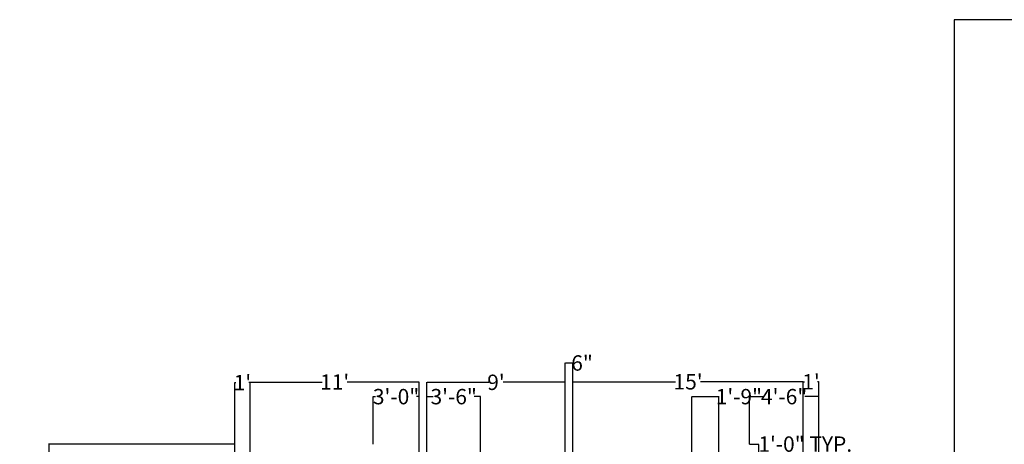
# Model space of a CAD drawing. Units: inches. Extents: x 2450 to 4494, y 1482 to 2597.
# Tile 3 of 7: x 2469 to 3238, y 2188 to 2519. Entities that reach past the tile are written whole.
import ezdxf

# ---------------------------------------------------------------- set-up
doc = ezdxf.new("R2010")
doc.units = ezdxf.units.IN
doc.header["$LTSCALE"] = 5
doc.header["$MEASUREMENT"] = 0
doc.layers.add('A-ANNO-DIMS', color=2, linetype='Continuous', lineweight=18)
doc.styles.get("Standard").update_dxf_attribs({"font": 'arial.ttf'})
doc.dimstyles.get("Standard").update_dxf_attribs({"dimtxt": 12, "dimasz": 0.18, "dimexe": 0.18, "dimexo": 0.0625, "dimgap": 0.09, "dimtad": 0, "dimtih": 1, "dimtoh": 1, "dimdec": 0, "dimzin": 0, "dimdsep": 46, "dimlunit": 3, "dimtxsty": 'Standard', "dimcen": 0.09, "dimadec": 0, "dimazin": 0, "dimtfac": 1, "dimtdec": 0, "dimtofl": 0, "dimtmove": 0, "dimatfit": 3, "dimfxl": 1, "dimtolj": 1, "dimtzin": 0, "dimarcsym": 0})

# ---------------------------------------------------------------- blocks, each defined once
blk = doc.blocks.new('*D6')
at = {"layer": 'A-ANNO-DIMS', "color": 0, "lineweight": -2, "ltscale": 5, "transparency": 16777216}
for p, q in [((2900.93, 2175.63), (2900.93, 2236.59)), ((2901.11, 2236.41), (2981.22, 2236.41)), ((3080.75, 2236.41), (3000.64, 2236.41)), ((3080.93, 2175.63), (3080.93, 2236.59))]:
    blk.add_line(p, q, dxfattribs=at)
at = {"layer": 'A-ANNO-DIMS', "color": 0, "ltscale": 5, "transparency": 16777216}
for points in [[(2901.11, 2236.44), (2901.11, 2236.38), (2900.93, 2236.41)], [(3080.75, 2236.44), (3080.75, 2236.38), (3080.93, 2236.41)]]:
    blk.add_solid(points, dxfattribs=at)
at = {"layer": 'Defpoints', "color": 0, "ltscale": 5, "transparency": 16777216}
for p in [(3080.93, 2236.41), (2900.93, 2175.57), (3080.93, 2175.57)]:
    blk.add_point(p, dxfattribs=at)
at = {"layer": 'A-ANNO-DIMS', "color": 0, "ltscale": 5, "transparency": 16777216, "insert": (2990.93, 2236.41), "char_height": 12, "attachment_point": 5}
blk.add_mtext("\\A1;15'", dxfattribs=at)
blk = doc.blocks.new('*D7')
at = {"layer": 'A-ANNO-DIMS', "color": 0, "lineweight": -2, "ltscale": 5, "transparency": 16777216}
for p, q in [((3080.93, 2175.63), (3080.93, 2236.59)), ((3081.11, 2236.41), (3081.88, 2236.41)), ((3092.75, 2236.41), (3091.98, 2236.41)), ((3092.93, 2175.63), (3092.93, 2236.59))]:
    blk.add_line(p, q, dxfattribs=at)
at = {"layer": 'A-ANNO-DIMS', "color": 0, "ltscale": 5, "transparency": 16777216}
for points in [[(3081.11, 2236.44), (3081.11, 2236.38), (3080.93, 2236.41)], [(3092.75, 2236.44), (3092.75, 2236.38), (3092.93, 2236.41)]]:
    blk.add_solid(points, dxfattribs=at)
at = {"layer": 'Defpoints', "color": 0, "ltscale": 5, "transparency": 16777216}
for p in [(3092.93, 2236.41), (3080.93, 2175.57), (3092.93, 2175.57)]:
    blk.add_point(p, dxfattribs=at)
at = {"layer": 'A-ANNO-DIMS', "color": 0, "ltscale": 5, "transparency": 16777216, "insert": (3086.93, 2236.41), "char_height": 12, "attachment_point": 5}
blk.add_mtext("\\A1;1'", dxfattribs=at)
blk = doc.blocks.new('*D8')
at = {"layer": 'A-ANNO-DIMS', "color": 0, "lineweight": -2, "ltscale": 5, "transparency": 16777216}
for p, q in [((2786.93, 2175.63), (2786.93, 2236.19)), ((2787.11, 2236.01), (2835.32, 2236.01)), ((2894.75, 2236.01), (2846.54, 2236.01)), ((2894.93, 2175.63), (2894.93, 2236.19))]:
    blk.add_line(p, q, dxfattribs=at)
at = {"layer": 'A-ANNO-DIMS', "color": 0, "ltscale": 5, "transparency": 16777216}
for points in [[(2787.11, 2236.04), (2787.11, 2235.98), (2786.93, 2236.01)], [(2894.75, 2236.04), (2894.75, 2235.98), (2894.93, 2236.01)]]:
    blk.add_solid(points, dxfattribs=at)
at = {"layer": 'Defpoints', "color": 0, "ltscale": 5, "transparency": 16777216}
for p in [(2894.93, 2236.01), (2786.93, 2175.57), (2894.93, 2175.57)]:
    blk.add_point(p, dxfattribs=at)
at = {"layer": 'A-ANNO-DIMS', "color": 0, "ltscale": 5, "transparency": 16777216, "insert": (2840.93, 2236.01), "char_height": 12, "attachment_point": 5}
blk.add_mtext("\\A1;9'", dxfattribs=at)
blk = doc.blocks.new('*D9')
at = {"layer": 'A-ANNO-DIMS', "color": 0, "lineweight": -2, "ltscale": 5, "transparency": 16777216}
for p, q in [((2894.93, 2175.63), (2894.93, 2251.28)), ((2895.11, 2251.1), (2900.75, 2251.1)), ((2900.93, 2175.63), (2900.93, 2251.28)), ((2900.93, 2251.1), (2901.11, 2251.1))]:
    blk.add_line(p, q, dxfattribs=at)
at = {"layer": 'A-ANNO-DIMS', "color": 0, "ltscale": 5, "transparency": 16777216}
for points in [[(2895.11, 2251.13), (2895.11, 2251.07), (2894.93, 2251.1)], [(2900.75, 2251.13), (2900.75, 2251.07), (2900.93, 2251.1)]]:
    blk.add_solid(points, dxfattribs=at)
at = {"layer": 'Defpoints', "color": 0, "ltscale": 5, "transparency": 16777216}
for p in [(2900.93, 2251.1), (2894.93, 2175.57), (2900.93, 2175.57)]:
    blk.add_point(p, dxfattribs=at)
at = {"layer": 'A-ANNO-DIMS', "color": 0, "ltscale": 5, "transparency": 16777216, "insert": (2908.13, 2251.1), "char_height": 12, "attachment_point": 5}
blk.add_mtext('\\A1;6"', dxfattribs=at)
blk = doc.blocks.new('*D10')
at = {"layer": 'A-ANNO-DIMS', "color": 0, "lineweight": -2, "ltscale": 5, "transparency": 16777216}
for p, q in [((2648.93, 2175.63), (2648.93, 2236.37)), ((2649.11, 2236.19), (2705.22, 2236.19)), ((2780.75, 2236.19), (2724.64, 2236.19)), ((2780.93, 2175.63), (2780.93, 2236.37))]:
    blk.add_line(p, q, dxfattribs=at)
at = {"layer": 'A-ANNO-DIMS', "color": 0, "ltscale": 5, "transparency": 16777216}
for points in [[(2649.11, 2236.22), (2649.11, 2236.16), (2648.93, 2236.19)], [(2780.75, 2236.22), (2780.75, 2236.16), (2780.93, 2236.19)]]:
    blk.add_solid(points, dxfattribs=at)
at = {"layer": 'Defpoints', "color": 0, "ltscale": 5, "transparency": 16777216}
for p in [(2780.93, 2236.19), (2648.93, 2175.57), (2780.93, 2175.57)]:
    blk.add_point(p, dxfattribs=at)
at = {"layer": 'A-ANNO-DIMS', "color": 0, "ltscale": 5, "transparency": 16777216, "insert": (2714.93, 2236.19), "char_height": 12, "attachment_point": 5}
blk.add_mtext("\\A1;11'", dxfattribs=at)
blk = doc.blocks.new('*D11')
at = {"layer": 'A-ANNO-DIMS', "color": 0, "lineweight": -2, "ltscale": 5, "transparency": 16777216}
for p, q in [((2636.93, 2175.63), (2636.93, 2235.95)), ((2637.11, 2235.77), (2637.88, 2235.77)), ((2648.75, 2235.77), (2647.98, 2235.77)), ((2648.93, 2175.63), (2648.93, 2235.95))]:
    blk.add_line(p, q, dxfattribs=at)
at = {"layer": 'A-ANNO-DIMS', "color": 0, "ltscale": 5, "transparency": 16777216}
for points in [[(2637.11, 2235.8), (2637.11, 2235.74), (2636.93, 2235.77)], [(2648.75, 2235.8), (2648.75, 2235.74), (2648.93, 2235.77)]]:
    blk.add_solid(points, dxfattribs=at)
at = {"layer": 'Defpoints', "color": 0, "ltscale": 5, "transparency": 16777216}
for p in [(2636.93, 2235.77), (2636.93, 2175.57), (2648.93, 2175.57)]:
    blk.add_point(p, dxfattribs=at)
at = {"layer": 'A-ANNO-DIMS', "color": 0, "ltscale": 5, "transparency": 16777216, "insert": (2642.93, 2235.77), "char_height": 12, "attachment_point": 5}
blk.add_mtext("\\A1;1'", dxfattribs=at)
blk = doc.blocks.new('*D41')
at = {"layer": 'A-ANNO-DIMS', "color": 0, "lineweight": -2, "ltscale": 5, "transparency": 16777216}
for p, q in [((2990.93, 2175.51), (2990.93, 2168.19)), ((2991.11, 2168.37), (3038.75, 2168.37)), ((3038.93, 2175.51), (3038.93, 2168.19)), ((3038.93, 2168.37), (3039.11, 2168.37))]:
    blk.add_line(p, q, dxfattribs=at)
at = {"layer": 'A-ANNO-DIMS', "color": 0, "ltscale": 5, "transparency": 16777216}
for points in [[(2991.11, 2168.4), (2991.11, 2168.34), (2990.93, 2168.37)], [(3038.75, 2168.4), (3038.75, 2168.34), (3038.93, 2168.37)]]:
    blk.add_solid(points, dxfattribs=at)
at = {"layer": 'Defpoints', "color": 0, "ltscale": 5, "transparency": 16777216}
for p in [(2990.93, 2175.57), (3038.93, 2175.57), (3038.93, 2168.37)]:
    blk.add_point(p, dxfattribs=at)
at = {"layer": 'A-ANNO-DIMS', "color": 0, "ltscale": 5, "transparency": 16777216, "insert": (3115.13, 2168.37), "char_height": 12, "attachment_point": 5}
blk.add_mtext('\\A1;WINDOW 4\'-0" TYP.', dxfattribs=at)
blk = doc.blocks.new('*D42')
at = {"layer": 'A-ANNO-DIMS', "color": 0, "lineweight": -2, "ltscale": 5, "transparency": 16777216}
for p, q in [((3038.99, 2187.57), (3046.31, 2187.57)), ((3046.13, 2187.57), (3046.13, 2187.75)), ((3046.13, 2187.75), (3046.31, 2187.75)), ((3046.13, 2175.75), (3046.13, 2187.39)), ((3038.99, 2175.57), (3046.31, 2175.57))]:
    blk.add_line(p, q, dxfattribs=at)
at = {"layer": 'A-ANNO-DIMS', "color": 0, "ltscale": 5, "transparency": 16777216}
for points in [[(3046.1, 2187.39), (3046.16, 2187.39), (3046.13, 2187.57)], [(3046.1, 2175.75), (3046.16, 2175.75), (3046.13, 2175.57)]]:
    blk.add_solid(points, dxfattribs=at)
at = {"layer": 'Defpoints', "color": 0, "ltscale": 5, "transparency": 16777216}
for p in [(3038.93, 2187.57), (3046.13, 2187.57), (3038.93, 2175.57)]:
    blk.add_point(p, dxfattribs=at)
at = {"layer": 'A-ANNO-DIMS', "color": 0, "ltscale": 5, "transparency": 16777216, "insert": (3082.41, 2187.75), "char_height": 12, "attachment_point": 5}
blk.add_mtext('\\A1;1\'-0" TYP.', dxfattribs=at)
blk = doc.blocks.new('*D70')
at = {"layer": 'A-ANNO-DIMS', "color": 0, "lineweight": -2, "ltscale": 5, "transparency": 16777216}
for p, q in [((2636.87, 2187.57), (2491.5, 2187.57)), ((2491.68, 2187.39), (2491.68, 1983.79)), ((2491.68, 1767.75), (2491.68, 1971.35)), ((2642.87, 1767.57), (2491.5, 1767.57))]:
    blk.add_line(p, q, dxfattribs=at)
at = {"layer": 'A-ANNO-DIMS', "color": 0, "ltscale": 5, "transparency": 16777216}
for points in [[(2491.65, 2187.39), (2491.71, 2187.39), (2491.68, 2187.57)], [(2491.65, 1767.75), (2491.71, 1767.75), (2491.68, 1767.57)]]:
    blk.add_solid(points, dxfattribs=at)
at = {"layer": 'Defpoints', "color": 0, "ltscale": 5, "transparency": 16777216}
for p in [(2636.93, 2187.57), (2491.68, 1767.57), (2642.93, 1767.57)]:
    blk.add_point(p, dxfattribs=at)
at = {"layer": 'A-ANNO-DIMS', "color": 0, "ltscale": 5, "transparency": 16777216, "insert": (2491.68, 1977.57), "char_height": 12, "attachment_point": 5}
blk.add_mtext('\\A1;35\'-0"', dxfattribs=at)
blk = doc.blocks.new('*D72')
at = {"layer": 'A-ANNO-DIMS', "color": 0, "lineweight": -2, "ltscale": 5, "transparency": 16777216}
for p, q in [((3426.23, 2519.27), (3198.61, 2519.27)), ((3198.79, 2519.09), (3198.79, 2045.48)), ((3198.79, 1559.45), (3198.79, 2033.05)), ((3426.23, 1559.27), (3198.61, 1559.27))]:
    blk.add_line(p, q, dxfattribs=at)
at = {"layer": 'A-ANNO-DIMS', "color": 0, "ltscale": 5, "transparency": 16777216}
for points in [[(3198.76, 2519.09), (3198.82, 2519.09), (3198.79, 2519.27)], [(3198.76, 1559.45), (3198.82, 1559.45), (3198.79, 1559.27)]]:
    blk.add_solid(points, dxfattribs=at)
at = {"layer": 'Defpoints', "color": 0, "ltscale": 5, "transparency": 16777216}
for p in [(3198.79, 2519.27), (3426.29, 2519.27), (3426.29, 1559.27)]:
    blk.add_point(p, dxfattribs=at)
at = {"layer": 'A-ANNO-DIMS', "color": 0, "ltscale": 5, "transparency": 16777216, "insert": (3198.79, 2039.27), "char_height": 12, "attachment_point": 5}
blk.add_mtext('\\A1;80\'-0"', dxfattribs=at)
blk = doc.blocks.new('*D75')
at = {"layer": 'A-ANNO-DIMS', "color": 0, "lineweight": -2, "ltscale": 5, "transparency": 16777216}
for p, q in [((2744.93, 2187.63), (2744.93, 2225)), ((2745.11, 2224.82), (2746.9, 2224.82)), ((2780.75, 2224.82), (2778.97, 2224.82)), ((2780.93, 2187.63), (2780.93, 2225))]:
    blk.add_line(p, q, dxfattribs=at)
at = {"layer": 'A-ANNO-DIMS', "color": 0, "ltscale": 5, "transparency": 16777216}
for points in [[(2745.11, 2224.85), (2745.11, 2224.79), (2744.93, 2224.82)], [(2780.75, 2224.85), (2780.75, 2224.79), (2780.93, 2224.82)]]:
    blk.add_solid(points, dxfattribs=at)
at = {"layer": 'Defpoints', "color": 0, "ltscale": 5, "transparency": 16777216}
for p in [(2780.93, 2224.82), (2744.93, 2187.57), (2780.93, 2187.57)]:
    blk.add_point(p, dxfattribs=at)
at = {"layer": 'A-ANNO-DIMS', "color": 0, "ltscale": 5, "transparency": 16777216, "insert": (2762.93, 2224.82), "char_height": 12, "attachment_point": 5}
blk.add_mtext('\\A1;3\'-0"', dxfattribs=at)
blk = doc.blocks.new('*D77')
at = {"layer": 'A-ANNO-DIMS', "color": 0, "lineweight": -2, "ltscale": 5, "transparency": 16777216}
for p, q in [((3038.93, 2187.63), (3038.93, 2225)), ((3039.11, 2224.82), (3049.65, 2224.82)), ((3092.75, 2224.82), (3082.21, 2224.82)), ((3092.93, 2187.63), (3092.93, 2225))]:
    blk.add_line(p, q, dxfattribs=at)
at = {"layer": 'A-ANNO-DIMS', "color": 0, "ltscale": 5, "transparency": 16777216}
for points in [[(3039.11, 2224.85), (3039.11, 2224.79), (3038.93, 2224.82)], [(3092.75, 2224.85), (3092.75, 2224.79), (3092.93, 2224.82)]]:
    blk.add_solid(points, dxfattribs=at)
at = {"layer": 'Defpoints', "color": 0, "ltscale": 5, "transparency": 16777216}
for p in [(3092.93, 2224.82), (3038.93, 2187.57), (3092.93, 2187.57)]:
    blk.add_point(p, dxfattribs=at)
at = {"layer": 'A-ANNO-DIMS', "color": 0, "ltscale": 5, "transparency": 16777216, "insert": (3065.93, 2224.82), "char_height": 12, "attachment_point": 5}
blk.add_mtext('\\A1;4\'-6"', dxfattribs=at)
blk = doc.blocks.new('*D79')
at = {"layer": 'A-ANNO-DIMS', "color": 0, "lineweight": -2, "ltscale": 5, "transparency": 16777216}
for p, q in [((2786.93, 1779.63), (2786.93, 2225)), ((2787.11, 2224.82), (2791.9, 2224.82)), ((2828.75, 2224.82), (2823.97, 2224.82)), ((2828.93, 1779.63), (2828.93, 2225))]:
    blk.add_line(p, q, dxfattribs=at)
at = {"layer": 'A-ANNO-DIMS', "color": 0, "ltscale": 5, "transparency": 16777216}
for points in [[(2787.11, 2224.85), (2787.11, 2224.79), (2786.93, 2224.82)], [(2828.75, 2224.85), (2828.75, 2224.79), (2828.93, 2224.82)]]:
    blk.add_solid(points, dxfattribs=at)
at = {"layer": 'Defpoints', "color": 0, "ltscale": 5, "transparency": 16777216}
for p in [(2828.93, 2224.82), (2786.93, 1779.57), (2828.93, 1779.57)]:
    blk.add_point(p, dxfattribs=at)
at = {"layer": 'A-ANNO-DIMS', "color": 0, "ltscale": 5, "transparency": 16777216, "insert": (2807.93, 2224.82), "char_height": 12, "attachment_point": 5}
blk.add_mtext('\\A1;3\'-6"', dxfattribs=at)
blk = doc.blocks.new('*D81')
at = {"layer": 'A-ANNO-DIMS', "color": 0, "lineweight": -2, "ltscale": 5, "transparency": 16777216}
for p, q in [((2993.93, 1839.63), (2993.93, 2225)), ((2994.11, 2224.82), (3014.75, 2224.82)), ((3014.93, 1839.63), (3014.93, 2225)), ((3014.93, 2224.82), (3015.11, 2224.82))]:
    blk.add_line(p, q, dxfattribs=at)
at = {"layer": 'A-ANNO-DIMS', "color": 0, "ltscale": 5, "transparency": 16777216}
for points in [[(2994.11, 2224.85), (2994.11, 2224.79), (2993.93, 2224.82)], [(3014.75, 2224.85), (3014.75, 2224.79), (3014.93, 2224.82)]]:
    blk.add_solid(points, dxfattribs=at)
at = {"layer": 'Defpoints', "color": 0, "ltscale": 5, "transparency": 16777216}
for p in [(3014.93, 2224.82), (2993.93, 1839.57), (3014.93, 1839.57)]:
    blk.add_point(p, dxfattribs=at)
at = {"layer": 'A-ANNO-DIMS', "color": 0, "ltscale": 5, "transparency": 16777216, "insert": (3030.59, 2224.82), "char_height": 12, "attachment_point": 5}
blk.add_mtext('\\A1;1\'-9"', dxfattribs=at)

msp = doc.modelspace()

# ---------------------------------------------------------------- dimensions: what is measured, and where the dimension line sits
at = {"layer": 'A-ANNO-DIMS', "ltscale": 5}
for base, p1, p2, picture, middle in [((3198.79, 2519.27), (3426.29, 1559.27), (3426.29, 2519.27), '*D72', (3198.79, 2039.27)), ((2491.68, 1767.57), (2636.93, 2187.57), (2642.93, 1767.57), '*D70', (2491.68, 1977.57))]:
    dim = msp.add_linear_dim(base=base, p1=p1, p2=p2, angle=90, dimstyle='Standard', override={"dimdec": 1, "dimlfac": 1, "dimrnd": 0, "dimzin": 1, "dimdsep": 46, "dimlunit": 4, "dimfrac": 2}, dxfattribs=at)
    dim.commit()
    dim.dimension.update_dxf_attribs({"geometry": picture, "text_midpoint": middle})
for base, p1, p2, override, picture, middle in [((2900.93, 2251.1), (2894.93, 2175.57), (2900.93, 2175.57), {"dimclrd": 0, "dimclre": 0, "dimclrt": 0}, '*D9', (2908.13, 2251.1)), ((2636.93, 2235.77), (2648.93, 2175.57), (2636.93, 2175.57), {"dimclrd": 0, "dimclre": 0, "dimclrt": 0}, '*D11', (2642.93, 2235.77)), ((2780.93, 2236.19), (2648.93, 2175.57), (2780.93, 2175.57), {"dimclrd": 0, "dimclre": 0, "dimclrt": 0}, '*D10', (2714.93, 2236.19)), ((2894.93, 2236.01), (2786.93, 2175.57), (2894.93, 2175.57), {"dimclrd": 0, "dimclre": 0, "dimclrt": 0}, '*D8', (2840.93, 2236.01)), ((3080.93, 2236.41), (2900.93, 2175.57), (3080.93, 2175.57), {"dimclrd": 0, "dimclre": 0, "dimclrt": 0}, '*D6', (2990.93, 2236.41)), ((3092.93, 2236.41), (3080.93, 2175.57), (3092.93, 2175.57), {"dimclrd": 0, "dimclre": 0, "dimclrt": 0}, '*D7', (3086.93, 2236.41)), ((2780.93, 2224.82), (2744.93, 2187.57), (2780.93, 2187.57), {"dimdec": 1, "dimlfac": 1, "dimrnd": 0, "dimzin": 1, "dimdsep": 46, "dimlunit": 4, "dimfrac": 2}, '*D75', (2762.93, 2224.82)), ((2828.93, 2224.82), (2786.93, 1779.57), (2828.93, 1779.57), {"dimdec": 1, "dimlfac": 1, "dimrnd": 0, "dimzin": 1, "dimdsep": 46, "dimlunit": 4, "dimfrac": 2}, '*D79', (2807.93, 2224.82)), ((3014.93, 2224.82), (2993.93, 1839.57), (3014.93, 1839.57), {"dimdec": 1, "dimlfac": 1, "dimrnd": 0, "dimzin": 1, "dimdsep": 46, "dimlunit": 4, "dimfrac": 2}, '*D81', (3030.59, 2224.82)), ((3092.93, 2224.82), (3038.93, 2187.57), (3092.93, 2187.57), {"dimdec": 1, "dimlfac": 1, "dimrnd": 0, "dimzin": 1, "dimdsep": 46, "dimlunit": 4, "dimfrac": 2}, '*D77', (3065.93, 2224.82))]:
    dim = msp.add_linear_dim(base=base, p1=p1, p2=p2, dimstyle='Standard', override=override, dxfattribs=at)
    dim.commit()
    dim.dimension.update_dxf_attribs({"geometry": picture, "text_midpoint": middle})
dim = msp.add_linear_dim(base=(3046.13, 2187.57), p1=(3038.93, 2175.57), p2=(3038.93, 2187.57), angle=90, text='<> TYP.', dimstyle='Standard', override={"dimdec": 1, "dimlfac": 1, "dimrnd": 0, "dimzin": 1, "dimdsep": 46, "dimlunit": 4, "dimfrac": 2}, dxfattribs=at)
dim.commit()
dim.dimension.update_dxf_attribs({"geometry": '*D42', "text_midpoint": (3082.41, 2187.75)})
dim = msp.add_linear_dim(base=(3038.93, 2168.37), p1=(2990.93, 2175.57), p2=(3038.93, 2175.57), text='WINDOW <> TYP.', dimstyle='Standard', override={"dimdec": 1, "dimlfac": 1, "dimrnd": 0, "dimzin": 1, "dimdsep": 46, "dimlunit": 4, "dimfrac": 2}, dxfattribs=at)
dim.commit()
dim.dimension.update_dxf_attribs({"geometry": '*D41', "text_midpoint": (3115.13, 2168.37)})

doc.saveas('drawing.dxf')
